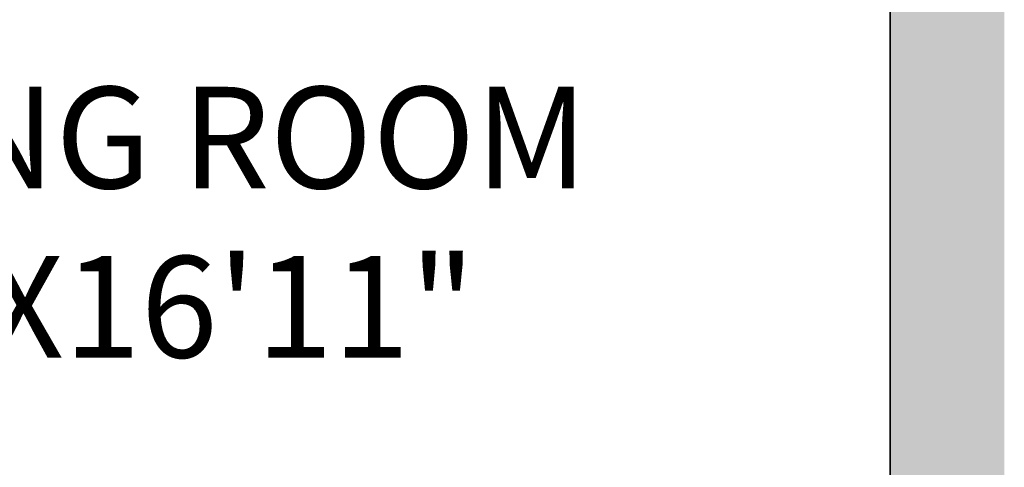
# Model space of a CAD drawing. Units: inches. Extents: x 3592 to 4861, y 1650 to 2243.
# Tile 4 of 30: x 4188 to 4265, y 1836 to 1872. Entities that reach past the tile are written whole.
import ezdxf

# ---------------------------------------------------------------- set-up
doc = ezdxf.new("R2010")
doc.units = ezdxf.units.IN
doc.layers.add('A-AREA-IDEN', color=7, linetype='Continuous', lineweight=18)
doc.layers.add('A-WALL', color=7, linetype='Continuous', lineweight=35)
doc.layers.add('A-WALL-PATT', color=252, linetype='Continuous', lineweight=13, true_color=0x939598)
doc.styles.get("Standard").update_dxf_attribs({"font": 'arial.ttf'})

msp = doc.modelspace()

# ---------------------------------------------------------------- hatches: boundary and pattern name
at = {"layer": 'A-WALL-PATT'}
h = msp.add_hatch(color=256, dxfattribs=at)
h.dxf.hatch_style = 1
h.paths.add_polyline_path([(4398.37, 2165.219), (4038.37, 2165.219), (4038.37, 1993.219), (4047.37, 1993.219), (4047.37, 2156.219), (4191.37, 2156.219), (4191.37, 2150.219), (4195.37, 2150.219), (4195.37, 2156.219), (4256.37, 2156.219), (4256.37, 2150.219), (4265.37, 2150.219), (4265.37, 2156.219), (4389.37, 2156.219), (4389.37, 2114.219), (4398.37, 2114.219)])
h.paths.add_polyline_path([(4265.37, 2102.219), (4256.37, 2102.219), (4256.37, 2096.219), (4195.37, 2096.219), (4195.37, 2102.219), (4191.37, 2102.219), (4191.37, 2020.219), (4195.37, 2020.219), (4195.37, 2087.219), (4256.37, 2087.219), (4256.37, 2020.219), (4306.37, 2020.219), (4306.37, 2024.219), (4265.37, 2024.219)], flags=17)
h.paths.add_polyline_path([(4398.37, 2066.219), (4389.37, 2066.219), (4389.37, 2024.219), (4348.37, 2024.219), (4348.37, 2020.219), (4389.37, 2020.219), (4389.37, 1989.719), (4398.37, 1989.719)])
h.paths.add_polyline_path([(4398.37, 1941.719), (4389.37, 1941.719), (4389.37, 1911.219), (4301.37, 1911.219), (4301.37, 1907.219), (4389.37, 1907.219), (4389.37, 1865.219), (4398.37, 1865.219)])
h.paths.add_polyline_path([(4398.37, 1817.219), (4389.37, 1817.219), (4389.37, 1775.219), (4265.37, 1775.219), (4265.37, 1911.219), (4256.37, 1911.219), (4256.37, 1817.219), (4220.87, 1817.219), (4220.87, 1808.219), (4256.37, 1808.219), (4256.37, 1766.219), (4389.37, 1766.219), (4389.37, 1694.219), (4256.37, 1694.219), (4256.37, 1685.219), (4398.37, 1685.219)])
h.paths.add_polyline_path([(4178.87, 1817.219), (4077.37, 1817.219), (4077.37, 1808.219), (4178.87, 1808.219)])
h.paths.add_polyline_path([(4111.37, 2020.219), (4155.37, 2020.219), (4155.37, 2024.219), (4077.37, 2024.219), (4077.37, 2020.219), (4107.37, 2020.219), (4107.37, 1942.219), (4047.37, 1942.219), (4047.37, 1969.219), (4038.37, 1969.219), (4038.37, 1911.219), (4047.37, 1911.219), (4047.37, 1938.219), (4107.37, 1938.219), (4107.37, 1860.219), (4077.37, 1860.219), (4077.37, 1856.219), (4111.37, 1856.219)])
h.paths.add_polyline_path([(4047.37, 1887.219), (4038.37, 1887.219), (4038.37, 1685.219), (4152.37, 1685.219), (4152.37, 1715.219), (4143.37, 1715.219), (4143.37, 1694.219), (4047.37, 1694.219)])
h.paths.add_polyline_path([(4152.37, 1772.219), (4143.37, 1772.219), (4143.37, 1751.219), (4152.37, 1751.219)], flags=17)

# ---------------------------------------------------------------- linework, layer by layer
at = {"layer": 'A-WALL'}
msp.add_line((4256.37, 1911.219), (4256.37, 1817.219), dxfattribs=at)

# ---------------------------------------------------------------- texts
at = {"layer": 'A-AREA-IDEN', "insert": (4148.844, 1866.23), "char_height": 8, "attachment_point": 1}
msp.add_mtext_dynamic_manual_height_columns('DRAWING ROOM\\P    12\'1"X16\'11"', width=142.74418, gutter_width=12.5, heights=[0], dxfattribs=at)

doc.saveas('drawing.dxf')
